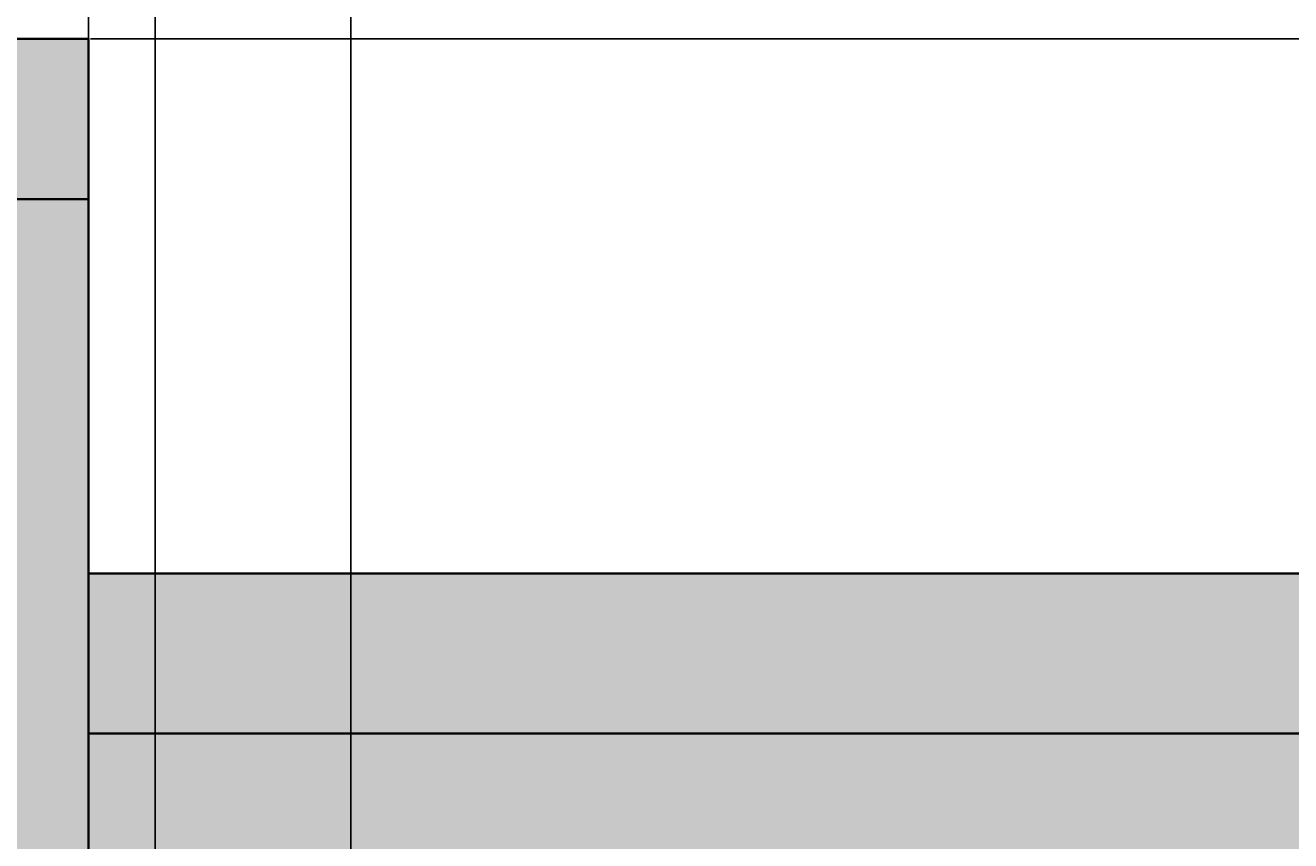
# Model space of a CAD drawing. Units: feet. Extents: x 2695 to 2912, y 795 to 1139.
# Tile 71 of 83: x 2769 to 2805, y 1100 to 1123. Entities that reach past the tile are written whole.
import ezdxf

# ---------------------------------------------------------------- set-up
doc = ezdxf.new("R2010")
doc.units = ezdxf.units.FT
for name, color, linetype, lineweight in [('A-ANNO-DIMS', 2, 'Continuous', 18), ('A-ELEV', 7, 'Continuous', 35), ('A-ELEV-PATT', 252, 'Continuous', 13)]:
    doc.layers.add(name, color=color, linetype=linetype, lineweight=lineweight)
doc.styles.get("Standard").update_dxf_attribs({"font": 'arial.ttf'})
doc.dimstyles.get("Standard").update_dxf_attribs({"dimtxt": 0.18, "dimasz": 0.18, "dimexe": 0.18, "dimexo": 0.0625, "dimgap": 0.09, "dimtad": 0, "dimtih": 1, "dimtoh": 1, "dimdec": 1, "dimzin": 0, "dimdsep": 46, "dimlunit": 3, "dimtxsty": 'Standard', "dimcen": 0.09, "dimadec": 0, "dimazin": 0, "dimtfac": 1, "dimtdec": 1, "dimtofl": 0, "dimtmove": 0, "dimatfit": 3, "dimfxl": 1, "dimtolj": 1, "dimtzin": 0, "dimarcsym": 0})

# ---------------------------------------------------------------- blocks, each defined once
blk = doc.blocks.new('*D8')
at = {"layer": 'A-ANNO-DIMS', "color": 0, "lineweight": -2, "transparency": 16777216}
for p, q in [((2715.885, 1050.373), (2715.885, 1138.886)), ((2716.065, 1138.706), (2742.866, 1138.706)), ((2770.456, 1138.706), (2743.655, 1138.706)), ((2770.636, 1122.993), (2770.636, 1138.886))]:
    blk.add_line(p, q, dxfattribs=at)
at = {"layer": 'A-ANNO-DIMS', "color": 0, "transparency": 16777216}
for points in [[(2716.065, 1138.736), (2716.065, 1138.676), (2715.885, 1138.706)], [(2770.456, 1138.736), (2770.456, 1138.676), (2770.636, 1138.706)]]:
    blk.add_solid(points, dxfattribs=at)
at = {"layer": 'Defpoints', "color": 0, "transparency": 16777216}
for p in [(2770.636, 1138.706), (2770.636, 1122.931), (2715.885, 1050.311)]:
    blk.add_point(p, dxfattribs=at)
at = {"layer": 'A-ANNO-DIMS', "color": 0, "transparency": 16777216, "insert": (2743.261, 1138.706), "char_height": 0.18, "attachment_point": 5}
blk.add_mtext('\\A1;54.75', dxfattribs=at)
blk = doc.blocks.new('*D9')
at = {"layer": 'A-ANNO-DIMS', "color": 0, "lineweight": -2, "transparency": 16777216}
for p, q in [((2770.636, 1122.993), (2770.636, 1138.886)), ((2770.816, 1138.706), (2773.942, 1138.706)), ((2777.854, 1138.706), (2774.728, 1138.706)), ((2778.034, 1020.886), (2778.034, 1138.886))]:
    blk.add_line(p, q, dxfattribs=at)
at = {"layer": 'A-ANNO-DIMS', "color": 0, "transparency": 16777216}
for points in [[(2770.816, 1138.736), (2770.816, 1138.676), (2770.636, 1138.706)], [(2777.854, 1138.736), (2777.854, 1138.676), (2778.034, 1138.706)]]:
    blk.add_solid(points, dxfattribs=at)
at = {"layer": 'Defpoints', "color": 0, "transparency": 16777216}
for p in [(2778.034, 1138.706), (2770.636, 1122.931), (2778.034, 1020.824)]:
    blk.add_point(p, dxfattribs=at)
at = {"layer": 'A-ANNO-DIMS', "color": 0, "transparency": 16777216, "insert": (2774.335, 1138.706), "char_height": 0.18, "attachment_point": 5}
blk.add_mtext('\\A1;7.398', dxfattribs=at)
blk = doc.blocks.new('*D10')
at = {"layer": 'A-ANNO-DIMS', "color": 0, "lineweight": -2, "transparency": 16777216}
for p, q in [((2778.034, 1020.886), (2778.034, 1138.886)), ((2778.214, 1138.706), (2810.411, 1138.706)), ((2843.395, 1138.706), (2811.198, 1138.706)), ((2843.575, 1020.886), (2843.575, 1138.886))]:
    blk.add_line(p, q, dxfattribs=at)
at = {"layer": 'A-ANNO-DIMS', "color": 0, "transparency": 16777216}
for points in [[(2778.214, 1138.736), (2778.214, 1138.676), (2778.034, 1138.706)], [(2843.395, 1138.736), (2843.395, 1138.676), (2843.575, 1138.706)]]:
    blk.add_solid(points, dxfattribs=at)
at = {"layer": 'Defpoints', "color": 0, "transparency": 16777216}
for p in [(2843.575, 1138.706), (2778.034, 1020.824), (2843.575, 1020.824)]:
    blk.add_point(p, dxfattribs=at)
at = {"layer": 'A-ANNO-DIMS', "color": 0, "transparency": 16777216, "insert": (2810.805, 1138.706), "char_height": 0.18, "attachment_point": 5}
blk.add_mtext('\\A1;65.54', dxfattribs=at)
blk = doc.blocks.new('*D22')
at = {"layer": 'A-ANNO-DIMS', "color": 0, "lineweight": -2, "transparency": 16777216}
for p, q in [((2770.699, 1122.931), (2911.424, 1122.931)), ((2911.244, 1122.751), (2911.244, 1115.565)), ((2911.244, 1108.015), (2911.244, 1115.201)), ((2895.532, 1107.835), (2911.424, 1107.835))]:
    blk.add_line(p, q, dxfattribs=at)
at = {"layer": 'A-ANNO-DIMS', "color": 0, "transparency": 16777216}
for points in [[(2911.214, 1122.751), (2911.274, 1122.751), (2911.244, 1122.931)], [(2911.214, 1108.015), (2911.274, 1108.015), (2911.244, 1107.835)]]:
    blk.add_solid(points, dxfattribs=at)
at = {"layer": 'Defpoints', "color": 0, "transparency": 16777216}
for p in [(2770.636, 1122.931), (2911.244, 1122.931), (2895.469, 1107.835)]:
    blk.add_point(p, dxfattribs=at)
at = {"layer": 'A-ANNO-DIMS', "color": 0, "transparency": 16777216, "insert": (2911.244, 1115.383), "char_height": 0.18, "attachment_point": 5}
blk.add_mtext('\\A1;15.095', dxfattribs=at)
blk = doc.blocks.new('*D48')
at = {"layer": 'A-ANNO-DIMS', "color": 0, "lineweight": -2, "transparency": 16777216}
for p, q in [((2770.636, 972.03), (2770.636, 1138.886)), ((2770.816, 1138.706), (2771.263, 1138.706)), ((2772.342, 1138.706), (2771.894, 1138.706)), ((2772.522, 972.03), (2772.522, 1138.886))]:
    blk.add_line(p, q, dxfattribs=at)
at = {"layer": 'A-ANNO-DIMS', "color": 0, "transparency": 16777216}
for points in [[(2770.816, 1138.736), (2770.816, 1138.676), (2770.636, 1138.706)], [(2772.342, 1138.736), (2772.342, 1138.676), (2772.522, 1138.706)]]:
    blk.add_solid(points, dxfattribs=at)
at = {"layer": 'Defpoints', "color": 0, "transparency": 16777216}
for p in [(2772.522, 1138.706), (2770.636, 971.967), (2772.522, 971.967)]:
    blk.add_point(p, dxfattribs=at)
at = {"layer": 'A-ANNO-DIMS', "color": 0, "transparency": 16777216, "insert": (2771.579, 1138.706), "char_height": 0.18, "attachment_point": 5}
blk.add_mtext('\\A1;1.89', dxfattribs=at)
blk = doc.blocks.new('*D49')
at = {"layer": 'A-ANNO-DIMS', "color": 0, "lineweight": -2, "transparency": 16777216}
for p, q in [((2772.522, 972.03), (2772.522, 1138.886)), ((2772.702, 1138.706), (2790.888, 1138.706)), ((2809.861, 1138.706), (2791.674, 1138.706)), ((2810.041, 972.03), (2810.041, 1138.886))]:
    blk.add_line(p, q, dxfattribs=at)
at = {"layer": 'A-ANNO-DIMS', "color": 0, "transparency": 16777216}
for points in [[(2772.702, 1138.736), (2772.702, 1138.676), (2772.522, 1138.706)], [(2809.861, 1138.736), (2809.861, 1138.676), (2810.041, 1138.706)]]:
    blk.add_solid(points, dxfattribs=at)
at = {"layer": 'Defpoints', "color": 0, "transparency": 16777216}
for p in [(2810.041, 1138.706), (2772.522, 971.967), (2810.041, 971.967)]:
    blk.add_point(p, dxfattribs=at)
at = {"layer": 'A-ANNO-DIMS', "color": 0, "transparency": 16777216, "insert": (2791.281, 1138.706), "char_height": 0.18, "attachment_point": 5}
blk.add_mtext('\\A1;37.52', dxfattribs=at)

msp = doc.modelspace()

# ---------------------------------------------------------------- hatches: boundary and pattern name
at = {"layer": 'A-ELEV-PATT'}
h = msp.add_hatch(color=256, dxfattribs=at)
h.set_gradient(color1=(255, 255, 255), tint=1)
h.paths.add_polyline_path([(2770.6361, 1122.9306), (2710.6361, 1122.9306), (2710.6361, 1118.4096), (2770.6361, 1118.4096)])
h.paths.add_polyline_path([(2890.6361, 1107.8588), (2770.6361, 1107.8588), (2770.6361, 1103.3378), (2890.6361, 1103.3378)])
h.paths.add_polyline_path([(2890.6361, 1062.9306), (2710.6361, 1062.9306), (2710.6361, 1056.9306), (2710.6361, 936.9306), (2710.6361, 924.3105), (2716.5358, 924.3105), (2890.6361, 924.3105), (2890.6361, 936.9306), (2715.8852, 936.9306), (2715.8852, 1050.3105), (2890.6361, 1050.3105)])
h.paths.add_polyline_path([(2716.5358, 924.3105), (2710.6361, 924.3105), (2710.6361, 810.9306), (2716.5358, 810.9306)])
h = msp.add_hatch(color=256, dxfattribs=at)
h.set_gradient(color1=(147, 149, 152), color2=(147, 149, 152), tint=1)
h.paths.add_polyline_path([(2770.6361, 1118.4096), (2710.6361, 1118.4096), (2710.6361, 1062.9306), (2770.6361, 1062.9306)])
h.paths.add_polyline_path([(2890.6361, 1103.3378), (2770.6361, 1103.3378), (2770.6361, 1062.9306), (2890.6361, 1062.9306)])
h.paths.add_polyline_path([(2730.7081, 1048.1052), (2755.1125, 1048.1052), (2755.1125, 936.9306), (2770.6361, 936.9306), (2770.6361, 1050.3105), (2715.8852, 1050.3105), (2715.8852, 936.9306), (2730.7081, 936.9306)])
h.paths.add_polyline_path([(2890.6361, 1050.3105), (2770.6361, 1050.3105), (2770.6361, 971.9673), (2778.0341, 971.9673), (2778.0341, 1020.8235), (2843.575, 1020.8235), (2843.575, 971.9673), (2890.6361, 971.9673)])
h.paths.add_polyline_path([(2888.1882, 970.7156), (2843.575, 970.7156), (2843.575, 964.8267), (2888.1882, 964.8267)])
h.paths.add_polyline_path([(2888.1882, 964.1328), (2843.575, 964.1328), (2843.575, 956.614), (2888.1882, 956.614)])
h.paths.add_polyline_path([(2888.1882, 955.9202), (2843.575, 955.9202), (2843.575, 949.2892), (2888.1882, 949.2892)])
h.paths.add_polyline_path([(2888.1882, 948.5954), (2843.575, 948.5954), (2843.575, 941.3507), (2888.1882, 941.3507)])
h.paths.add_polyline_path([(2888.1882, 940.6569), (2843.575, 940.6569), (2843.575, 936.9306), (2888.1882, 936.9306)])
h.paths.add_polyline_path([(2890.6361, 970.7156), (2888.9368, 970.7156), (2888.9368, 964.8267), (2890.6361, 964.8267)])
h.paths.add_polyline_path([(2890.6361, 964.1328), (2888.9368, 964.1328), (2888.9368, 956.614), (2890.6361, 956.614)])
h.paths.add_polyline_path([(2890.6361, 955.9202), (2888.9368, 955.9202), (2888.9368, 949.2892), (2890.6361, 949.2892)])
h.paths.add_polyline_path([(2890.6361, 940.6569), (2888.9368, 940.6569), (2888.9368, 936.9306), (2890.6361, 936.9306)])
h.paths.add_polyline_path([(2890.6361, 948.5954), (2888.9368, 948.5954), (2888.9368, 941.3507), (2890.6361, 941.3507)])
h.paths.add_polyline_path([(2772.5216, 970.7156), (2770.6361, 970.7156), (2770.6361, 964.8267), (2772.5216, 964.8267)])
h.paths.add_polyline_path([(2772.5216, 964.1328), (2770.6361, 964.1328), (2770.6361, 956.614), (2772.5216, 956.614)])
h.paths.add_polyline_path([(2772.5216, 955.9202), (2770.6361, 955.9202), (2770.6361, 949.2892), (2772.5216, 949.2892)])
h.paths.add_polyline_path([(2772.5216, 948.5954), (2770.6361, 948.5954), (2770.6361, 941.3507), (2772.5216, 941.3507)])
h.paths.add_polyline_path([(2772.5216, 940.6569), (2770.6361, 940.6569), (2770.6361, 936.9306), (2772.5216, 936.9306)])
h.paths.add_polyline_path([(2778.0341, 940.6569), (2773.2702, 940.6569), (2773.2702, 936.9306), (2778.0341, 936.9306)])
h.paths.add_polyline_path([(2778.0341, 970.7156), (2773.2702, 970.7156), (2773.2702, 964.8267), (2778.0341, 964.8267)])
h.paths.add_polyline_path([(2778.0341, 964.1328), (2773.2702, 964.1328), (2773.2702, 956.614), (2778.0341, 956.614)])
h.paths.add_polyline_path([(2778.0341, 955.9202), (2773.2702, 955.9202), (2773.2702, 949.2892), (2778.0341, 949.2892)])
h.paths.add_polyline_path([(2778.0341, 948.5954), (2773.2702, 948.5954), (2773.2702, 941.3507), (2778.0341, 941.3507)])
h.paths.add_polyline_path([(2810.0407, 940.6569), (2780.0341, 940.6569), (2780.0341, 936.9306), (2810.0407, 936.9306)])
h.paths.add_polyline_path([(2890.6361, 924.3105), (2770.6361, 924.3105), (2770.6361, 810.9306), (2773.5029, 810.9306), (2773.5029, 905.5143), (2805.9398, 905.5143), (2838.3767, 905.5143), (2838.3767, 810.9306), (2890.6361, 810.9306)])
h = msp.add_hatch(color=256, dxfattribs=at)
h.set_gradient(color1=(199, 200, 202), color2=(213, 227, 240), centered=1)
h.paths.add_polyline_path([(2890.6361, 1103.3378), (2770.6361, 1103.3378), (2770.6361, 1062.9306), (2890.6361, 1062.9306)])

# ---------------------------------------------------------------- linework, layer by layer
at = {"layer": 'A-ELEV'}
for p, q in [((2710.6361, 1122.9306), (2770.6361, 1122.9306)), ((2770.6361, 1122.9306), (2710.6361, 1122.9306)), ((2770.6361, 1122.9306), (2770.6361, 1062.9306)), ((2770.6361, 1107.8588), (2770.6361, 1122.9306)), ((2710.6361, 1118.4096), (2770.6361, 1118.4096)), ((2770.6361, 1118.4096), (2770.6361, 1103.3378)), ((2770.6361, 1107.8588), (2890.6361, 1107.8588)), ((2895.4694, 1107.8352), (2770.6361, 1107.8588)), ((2770.6361, 1103.3378), (2895.4694, 1103.3378))]:
    msp.add_line(p, q, dxfattribs=at)
for points in [[(2710.6361, 1118.4096), (2770.6361, 1118.4096)], [(2770.6361, 1103.3378), (2890.6361, 1103.3378)]]:
    msp.add_lwpolyline(points, dxfattribs=at)

# ---------------------------------------------------------------- dimensions: what is measured, and where the dimension line sits
at = {"layer": 'A-ANNO-DIMS'}
for base, p1, p2, override, picture, middle in [((2770.6361, 1138.7056), (2715.8852, 1050.3105), (2770.6361, 1122.9306), {"dimdec": 2, "dimlfac": 1, "dimrnd": 0, "dimzin": 0, "dimdsep": 46, "dimlunit": 2}, '*D8', (2743.2606, 1138.7056)), ((2778.0341, 1138.7056), (2770.6361, 1122.9306), (2778.0341, 1020.8235), {"dimdec": 3, "dimlfac": 1, "dimrnd": 0, "dimzin": 0, "dimdsep": 46, "dimlunit": 2}, '*D9', (2774.3351, 1138.7056)), ((2772.5216, 1138.7056), (2770.6361, 971.9673), (2772.5216, 971.9673), {"dimdec": 2, "dimlfac": 1, "dimrnd": 0, "dimzin": 0, "dimdsep": 46, "dimlunit": 2}, '*D48', (2771.5788, 1138.7056)), ((2810.0407, 1138.7056), (2772.5216, 971.9673), (2810.0407, 971.9673), {"dimdec": 2, "dimlfac": 1, "dimrnd": 0, "dimzin": 0, "dimdsep": 46, "dimlunit": 2}, '*D49', (2791.2811, 1138.7056)), ((2843.575, 1138.7056), (2778.0341, 1020.8235), (2843.575, 1020.8235), {"dimdec": 2, "dimlfac": 1, "dimrnd": 0, "dimzin": 0, "dimdsep": 46, "dimlunit": 2}, '*D10', (2810.8045, 1138.7056))]:
    dim = msp.add_linear_dim(base=base, p1=p1, p2=p2, dimstyle='Standard', override=override, dxfattribs=at)
    dim.commit()
    dim.dimension.update_dxf_attribs({"geometry": picture, "text_midpoint": middle})
dim = msp.add_linear_dim(base=(2911.2444, 1122.9306), p1=(2895.4694, 1107.8352), p2=(2770.6361, 1122.9306), angle=90, dimstyle='Standard', override={"dimdec": 3, "dimlfac": 1, "dimrnd": 0, "dimzin": 0, "dimdsep": 46, "dimlunit": 2}, dxfattribs=at)
dim.commit()
dim.dimension.update_dxf_attribs({"geometry": '*D22', "text_midpoint": (2911.2444, 1115.3829)})

doc.saveas('drawing.dxf')
